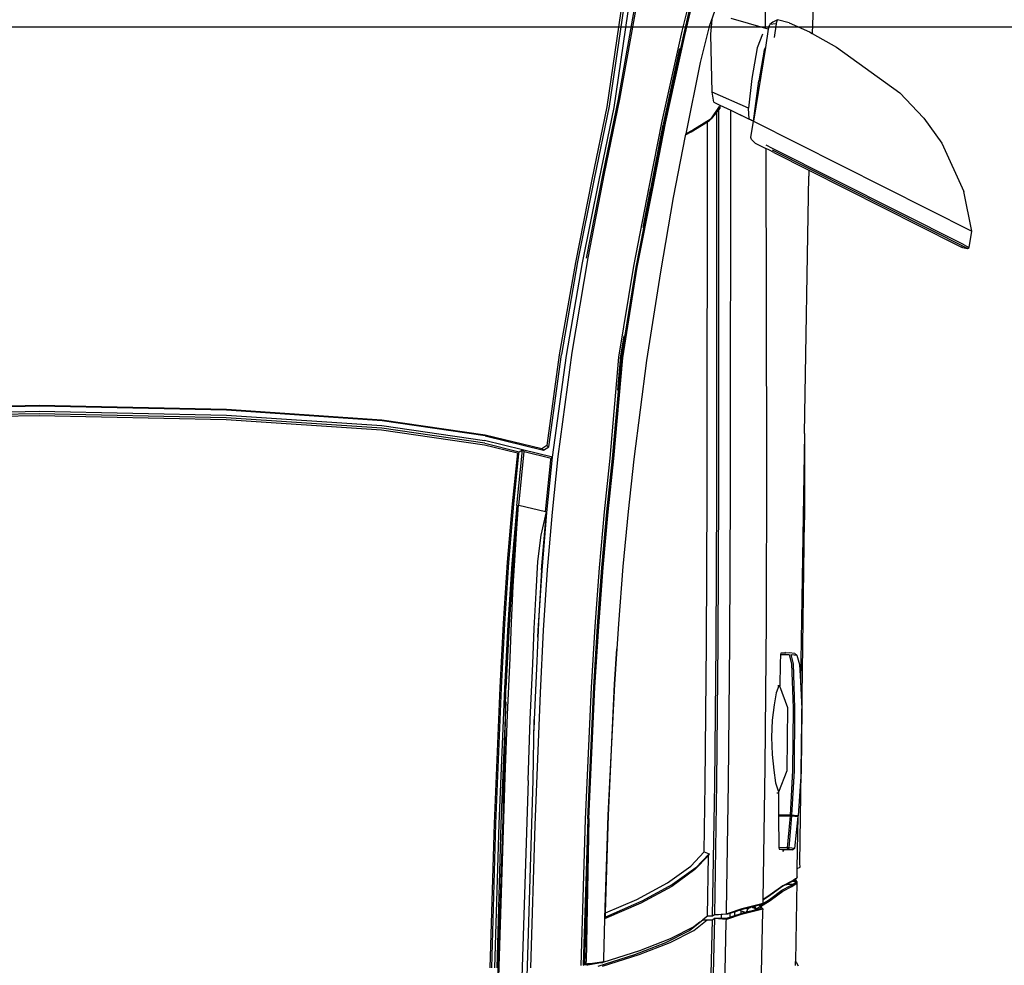
# Model space of a CAD drawing. Units: inches. Extents: x 1319 to 2030, y 219 to 1069.
# Tile 12 of 28: x 1461 to 1506, y 430 to 473. Entities that reach past the tile are written whole.
import ezdxf

# ---------------------------------------------------------------- set-up
doc = ezdxf.new("R2010")
doc.units = ezdxf.units.IN
doc.header["$MEASUREMENT"] = 0
doc.layers.get('0').update_dxf_attribs({"color": 12})
doc.layers.add('A-ANNO-DIMS', color=2, linetype='Continuous', lineweight=18)
doc.layers.add('C-PRKG-VEHC', color=8, linetype='Continuous', lineweight=13)
doc.layers.add('Edges', color=250, linetype='Continuous')
doc.styles.get("Standard").update_dxf_attribs({"font": 'arial.ttf'})
doc.dimstyles.get("Standard").update_dxf_attribs({"dimtxt": 7, "dimasz": 0.18, "dimexe": 0.18, "dimexo": 0.0625, "dimgap": 0.09, "dimtad": 0, "dimtih": 1, "dimtoh": 1, "dimzin": 0, "dimdsep": 46, "dimlunit": 3, "dimtxsty": 'Standard', "dimcen": 0.09, "dimadec": 0, "dimazin": 0, "dimtfac": 1, "dimtofl": 0, "dimtmove": 0, "dimatfit": 3, "dimfxl": 1, "dimtolj": 1, "dimtzin": 0, "dimarcsym": 0})

# ---------------------------------------------------------------- blocks, each defined once
blk = doc.blocks.new('Nissan Qashqai pl')
at = {"layer": 'Edges'}
for p, q in [((8.8918, 12.7444), (9.0186, 12.9956)), ((9.0386, 12.9907), (8.9254, 12.7664)), ((9.0186, 12.9956), (8.9731, 12.9865)), ((9.0374, 12.9925), (9.0186, 12.9956)), ((9.0356, 12.9888), (9.0374, 12.9925)), ((9.0386, 12.9907), (9.0374, 12.9925)), ((9.0376, 12.985), (9.0386, 12.9907)), ((8.9173, 12.961), (8.9731, 12.9865)), ((9.0333, 12.9845), (8.9232, 12.7662)), ((8.9483, 12.8082), (9.0343, 12.9785)), ((9.0356, 12.9888), (9.0333, 12.9845)), ((9.0343, 12.9785), (9.0347, 12.9794)), ((9.0347, 12.9794), (9.0362, 12.9822)), ((9.0362, 12.9822), (9.037, 12.9838)), ((9.0371, 12.9841), (9.037, 12.9838)), ((9.0371, 12.9841), (9.0376, 12.985)), ((9.0376, 12.985), (9.0371, 12.9847)), ((8.8885, 12.9405), (8.9173, 12.961)), ((8.8591, 12.9127), (8.8879, 12.94)), ((8.8885, 12.9405), (8.8879, 12.94)), ((8.8066, 12.84), (8.8591, 12.9127)), ((8.7908, 12.812), (8.8066, 12.84)), ((8.7222, 12.8144), (8.7908, 12.812)), ((8.7785, 12.7855), (8.7891, 12.8089)), ((8.7891, 12.8089), (8.7908, 12.812)), ((8.928, 12.7679), (8.9483, 12.8082)), ((8.9483, 12.8082), (8.9552, 12.8081)), ((9.2517, 12.8031), (8.9552, 12.8081)), ((9.2517, 12.8031), (9.351, 12.803)), ((9.2517, 12.8031), (9.5372, 12.7983)), ((9.641, 12.7991), (9.351, 12.803)), ((9.5069, 12.7941), (9.5176, 12.7972)), ((9.5176, 12.7972), (9.5372, 12.7983)), ((9.5372, 12.7983), (9.5689, 12.7999)), ((9.5689, 12.7999), (9.641, 12.7991)), ((9.641, 12.7991), (9.6921, 12.7956)), ((9.7466, 12.7978), (9.641, 12.7991)), ((9.7511, 12.7979), (9.7466, 12.7978)), ((9.7526, 12.7946), (9.7511, 12.7979)), ((9.5052, 12.7918), (9.5044, 12.7856)), ((9.5052, 12.7918), (9.5069, 12.7941)), ((9.5061, 12.7878), (9.5069, 12.7941)), ((9.5168, 12.7904), (9.5061, 12.7878)), ((9.5061, 12.7856), (9.5167, 12.7883)), ((9.5167, 12.7883), (9.5679, 12.7899)), ((9.5679, 12.792), (9.5168, 12.7904)), ((9.6401, 12.7914), (9.5679, 12.792)), ((9.5679, 12.7899), (9.64, 12.7892)), ((9.64, 12.7892), (9.6912, 12.7865)), ((9.6913, 12.7886), (9.6401, 12.7914)), ((9.6913, 12.7886), (9.6912, 12.7865)), ((9.6912, 12.7865), (9.6912, 12.7811)), ((9.692, 12.7943), (9.6913, 12.7886)), ((9.6921, 12.7956), (9.692, 12.7943)), ((9.6922, 12.7943), (9.692, 12.7943)), ((9.692, 12.7811), (9.6921, 12.7864)), ((9.6922, 12.7943), (9.6921, 12.7956)), ((9.7526, 12.7946), (9.6921, 12.7956)), ((9.6922, 12.7885), (9.6921, 12.7864)), ((9.6921, 12.7864), (9.7288, 12.7832)), ((9.6922, 12.7885), (9.693, 12.7955)), ((9.6922, 12.7885), (9.6922, 12.7943)), ((9.7288, 12.7854), (9.6922, 12.7885)), ((9.693, 12.7955), (9.7296, 12.7914)), ((9.7296, 12.7914), (9.7288, 12.7854)), ((9.7296, 12.7914), (9.7314, 12.7895)), ((9.7306, 12.7834), (9.7314, 12.7895)), ((9.7314, 12.7895), (9.7313, 12.7798)), ((9.7623, 12.7945), (9.7526, 12.7946)), ((9.7623, 12.7945), (9.7643, 12.7937)), ((9.7643, 12.7937), (9.7652, 12.7927)), ((9.7643, 12.7937), (9.7648, 12.7929)), ((9.7648, 12.7929), (9.7648, 12.7929)), ((9.7648, 12.7929), (9.7664, 12.7902)), ((9.7652, 12.7927), (9.7665, 12.7907)), ((9.7665, 12.7904), (9.7664, 12.7902)), ((9.7664, 12.7902), (9.7674, 12.7885)), ((9.7667, 12.7933), (9.7665, 12.7907)), ((9.7665, 12.7907), (9.7676, 12.7889)), ((9.7677, 12.7944), (9.7667, 12.7933)), ((9.7676, 12.7931), (9.7667, 12.7933)), ((9.7673, 12.7899), (9.7676, 12.7931)), ((9.7673, 12.7897), (9.7673, 12.7899)), ((9.7673, 12.7897), (9.7676, 12.7889)), ((9.7674, 12.7885), (9.7728, 12.7781)), ((9.769, 12.7926), (9.7676, 12.7931)), ((9.7676, 12.7889), (9.7684, 12.7875)), ((9.7676, 12.7887), (9.7678, 12.7882)), ((9.7677, 12.7944), (9.7677, 12.7944)), ((9.77, 12.7936), (9.7677, 12.7944)), ((9.7677, 12.7944), (9.8598, 12.7928)), ((9.7684, 12.7875), (9.7717, 12.781)), ((9.7712, 12.7892), (9.769, 12.7926)), ((9.7734, 12.7884), (9.77, 12.7936)), ((9.7707, 12.7848), (9.7709, 12.7893)), ((9.7709, 12.7893), (9.7712, 12.7892)), ((9.7724, 12.7874), (9.7712, 12.7892)), ((9.7778, 12.777), (9.7724, 12.7874)), ((9.7788, 12.778), (9.7734, 12.7884)), ((9.8598, 12.7928), (9.8614, 12.7937)), ((9.8643, 12.7927), (9.8598, 12.7928)), ((9.8614, 12.7937), (9.8647, 12.7956)), ((8.7785, 12.7855), (8.7751, 12.7719)), ((9.5037, 12.7806), (9.5045, 12.7814)), ((9.5044, 12.7856), (9.5045, 12.7814)), ((9.5045, 12.7814), (9.5045, 12.7759)), ((9.5045, 12.7759), (9.5063, 12.7755)), ((9.5063, 12.7755), (9.5061, 12.7856)), ((9.5063, 12.7755), (9.5168, 12.7751)), ((9.5168, 12.7751), (9.5423, 12.7746)), ((9.5423, 12.7746), (9.5422, 12.7736)), ((9.5426, 12.7747), (9.5423, 12.7746)), ((9.5426, 12.7747), (9.5424, 12.7735)), ((9.5678, 12.7837), (9.5426, 12.7747)), ((9.64, 12.7831), (9.5678, 12.7837)), ((9.6645, 12.7737), (9.64, 12.7831)), ((9.6912, 12.7811), (9.6911, 12.7796)), ((9.6911, 12.7796), (9.6911, 12.7732)), ((9.692, 12.7811), (9.6912, 12.7811)), ((9.692, 12.7796), (9.692, 12.7811)), ((9.692, 12.7733), (9.692, 12.7796)), ((9.7288, 12.7832), (9.7287, 12.7734)), ((9.7306, 12.7834), (9.7288, 12.7854)), ((9.7288, 12.7854), (9.7288, 12.7832)), ((9.7288, 12.7832), (9.7306, 12.7834)), ((9.7305, 12.7738), (9.7306, 12.7834)), ((9.7305, 12.7738), (9.7313, 12.7798)), ((9.733, 12.7782), (9.7313, 12.7798)), ((9.7717, 12.781), (9.7707, 12.7848)), ((9.7717, 12.781), (9.7738, 12.7771)), ((9.7728, 12.7781), (9.7832, 12.7637)), ((9.7738, 12.7771), (9.7842, 12.7627)), ((9.7883, 12.7626), (9.7778, 12.777)), ((9.7894, 12.7636), (9.7788, 12.778)), ((8.7751, 12.7719), (8.7779, 12.7668)), ((8.7798, 12.7703), (8.7751, 12.7719)), ((8.7779, 12.7668), (8.7807, 12.763)), ((8.7798, 12.7703), (8.7807, 12.763)), ((8.7798, 12.7703), (8.7954, 12.7683)), ((8.7849, 12.7615), (8.7807, 12.763)), ((8.9232, 12.7662), (8.9194, 12.7588)), ((8.928, 12.7679), (8.925, 12.762)), ((9.5422, 12.7736), (9.5422, 12.7725)), ((9.5422, 12.7736), (9.5424, 12.7735)), ((9.5424, 12.7735), (9.5503, 12.7706)), ((9.5503, 12.7706), (9.5641, 12.7681)), ((9.5641, 12.7681), (9.5818, 12.766)), ((9.5818, 12.766), (9.6016, 12.7651)), ((9.6016, 12.7651), (9.6215, 12.766)), ((9.6215, 12.766), (9.6395, 12.7676)), ((9.6395, 12.7676), (9.654, 12.7697)), ((9.654, 12.7697), (9.6633, 12.7726)), ((9.6633, 12.7726), (9.6645, 12.7737)), ((9.6655, 12.7733), (9.6645, 12.7737)), ((9.6655, 12.7733), (9.6911, 12.7732)), ((9.6655, 12.7713), (9.6655, 12.7733)), ((9.6911, 12.7732), (9.692, 12.7733)), ((9.692, 12.7733), (9.7287, 12.7734)), ((9.7287, 12.7734), (9.7305, 12.7738)), ((9.7832, 12.7637), (9.7887, 12.7552)), ((9.7965, 12.7526), (9.7894, 12.7636)), ((8.7849, 12.7582), (8.7205, 12.7579)), ((8.7734, 12.7181), (8.7849, 12.7582)), ((8.7849, 12.7615), (8.7858, 12.7613)), ((8.7849, 12.7582), (8.7856, 12.7608)), ((8.7858, 12.7613), (8.7856, 12.7608)), ((8.7858, 12.7613), (8.807, 12.758)), ((8.7917, 12.7547), (8.8075, 12.7486)), ((8.8102, 12.7568), (8.807, 12.758)), ((8.807, 12.758), (8.8918, 12.7444)), ((8.8102, 12.7568), (8.8455, 12.7506)), ((8.9171, 12.7464), (8.9233, 12.7586)), ((8.925, 12.762), (8.9233, 12.7586)), ((8.9233, 12.7586), (9.2886, 12.7594)), ((9.2886, 12.7594), (9.4673, 12.7589)), ((9.4673, 12.7589), (9.6358, 12.7575)), ((9.6358, 12.7575), (9.7887, 12.7552)), ((9.7842, 12.7627), (9.7891, 12.7552)), ((9.7933, 12.7549), (9.7883, 12.7626)), ((9.7887, 12.7552), (9.7891, 12.7552)), ((9.7891, 12.7552), (9.79, 12.7552)), ((9.79, 12.7552), (9.7931, 12.7552)), ((9.7931, 12.7552), (9.7934, 12.7535)), ((9.7931, 12.7552), (9.7933, 12.7549)), ((9.7933, 12.7549), (9.7941, 12.7541)), ((9.7934, 12.7535), (9.7938, 12.7538)), ((9.7934, 12.7535), (9.7937, 12.7524)), ((9.7937, 12.7524), (9.7992, 12.7308)), ((9.7941, 12.7541), (9.7943, 12.7535)), ((9.7955, 12.7516), (9.7943, 12.7535)), ((9.7943, 12.7535), (9.7964, 12.7453)), ((9.7963, 12.7523), (9.7955, 12.7516)), ((9.7963, 12.7523), (9.7963, 12.7524)), ((9.7964, 12.7524), (9.7963, 12.7523)), ((9.7992, 12.7476), (9.7963, 12.7523)), ((9.7967, 12.7526), (9.7964, 12.7524)), ((9.7964, 12.7525), (9.7964, 12.7524)), ((9.7964, 12.7524), (9.7996, 12.7475)), ((9.7983, 12.7541), (9.7965, 12.7526)), ((9.7965, 12.7526), (9.7967, 12.7526)), ((9.7977, 12.7535), (9.7967, 12.7526)), ((9.7967, 12.7526), (9.7986, 12.7526)), ((9.7982, 12.754), (9.7977, 12.7535)), ((9.7983, 12.7541), (9.7982, 12.754)), ((9.7986, 12.7526), (9.7982, 12.754)), ((9.7986, 12.7544), (9.7983, 12.7541)), ((9.7993, 12.755), (9.7986, 12.7544)), ((9.7988, 12.7516), (9.7986, 12.7526)), ((9.7998, 12.7477), (9.7988, 12.7516)), ((9.7999, 12.7522), (9.7993, 12.755)), ((9.7993, 12.755), (9.8024, 12.7549)), ((9.8054, 12.7307), (9.7999, 12.7522)), ((9.8024, 12.7549), (9.9426, 12.7518)), ((8.8075, 12.7486), (8.8429, 12.7426)), ((8.8429, 12.7426), (8.8771, 12.7388)), ((8.8918, 12.7444), (8.8455, 12.7506)), ((8.8815, 12.7228), (8.892, 12.7444)), ((8.8908, 12.7421), (8.8895, 12.7393)), ((8.8906, 12.7418), (8.8895, 12.7393)), ((8.8906, 12.7418), (8.8911, 12.7428)), ((8.892, 12.7444), (8.8908, 12.7421)), ((8.8911, 12.7428), (8.8919, 12.7444)), ((8.8911, 12.7428), (8.8919, 12.7444)), ((8.8919, 12.7444), (8.8911, 12.7428)), ((8.8919, 12.7444), (8.8918, 12.7444)), ((8.892, 12.7444), (8.8919, 12.7444)), ((8.8919, 12.7444), (8.8919, 12.7444)), ((8.8919, 12.7444), (8.8919, 12.7444)), ((8.9106, 12.7413), (8.892, 12.7444)), ((8.892, 12.7444), (8.892, 12.7444)), ((8.9131, 12.7421), (8.9106, 12.7413)), ((8.9171, 12.7464), (8.9131, 12.7421)), ((8.9171, 12.7464), (8.917, 12.7468)), ((9.7964, 12.7453), (9.7992, 12.7476)), ((9.7964, 12.7453), (9.7973, 12.7418)), ((9.7977, 12.7431), (9.7973, 12.7418)), ((9.7973, 12.7418), (9.7977, 12.7409)), ((9.7973, 12.7418), (9.7977, 12.7399)), ((9.7977, 12.7444), (9.7985, 12.7451)), ((9.7985, 12.7451), (9.7977, 12.7431)), ((9.7977, 12.7431), (9.7977, 12.7444)), ((9.7977, 12.7399), (9.7977, 12.7409)), ((9.7977, 12.7409), (9.7987, 12.7388)), ((9.7989, 12.7461), (9.7985, 12.7451)), ((9.7998, 12.7466), (9.7989, 12.7461)), ((9.7998, 12.7466), (9.7992, 12.7476)), ((9.7996, 12.7475), (9.7998, 12.7477)), ((9.8002, 12.7461), (9.7996, 12.7475)), ((9.8001, 12.7468), (9.7996, 12.7475)), ((9.8001, 12.7468), (9.7998, 12.7477)), ((9.8003, 12.7458), (9.7998, 12.7466)), ((9.8002, 12.7461), (9.8001, 12.7468)), ((9.8003, 12.7458), (9.8002, 12.7461)), ((9.8027, 12.7364), (9.8003, 12.7458)), ((8.8771, 12.7388), (8.8585, 12.6969)), ((8.8895, 12.7393), (8.8771, 12.7388)), ((8.8815, 12.7228), (8.8895, 12.7393)), ((9.7977, 12.7399), (9.7978, 12.7397)), ((9.7987, 12.7388), (9.7978, 12.7397)), ((9.7978, 12.7397), (9.7987, 12.7362)), ((9.7987, 12.7388), (9.7992, 12.7377)), ((9.7987, 12.7362), (9.7992, 12.7377)), ((9.7987, 12.7362), (9.8002, 12.7301)), ((9.7992, 12.7377), (9.8027, 12.7364)), ((9.7992, 12.7308), (9.8044, 12.7151)), ((9.8002, 12.7301), (9.8008, 12.7285)), ((9.8008, 12.7285), (9.8014, 12.7303)), ((9.8014, 12.7303), (9.8031, 12.7349)), ((9.8043, 12.7303), (9.8014, 12.7303)), ((9.8031, 12.7349), (9.8027, 12.7364)), ((9.8043, 12.7303), (9.8031, 12.7349)), ((9.8044, 12.73), (9.8043, 12.7303)), ((9.8067, 12.7229), (9.8044, 12.73)), ((9.8106, 12.715), (9.8054, 12.7307)), ((8.8734, 12.7057), (8.8793, 12.7181)), ((8.8793, 12.7181), (8.8815, 12.7228)), ((9.3194, 12.7179), (8.8793, 12.7181)), ((9.4919, 12.7173), (9.3194, 12.7179)), ((9.8008, 12.7285), (9.8014, 12.7265)), ((9.8014, 12.7265), (9.803, 12.723)), ((9.8014, 12.7265), (9.8026, 12.723)), ((9.803, 12.723), (9.8026, 12.723)), ((9.8026, 12.723), (9.8046, 12.7171)), ((9.8067, 12.7229), (9.803, 12.723)), ((9.8086, 12.7171), (9.8067, 12.7229)), ((9.6538, 12.7157), (9.4919, 12.7173)), ((9.802, 12.7133), (9.6538, 12.7157)), ((9.8051, 12.7132), (9.802, 12.7133)), ((9.8044, 12.7151), (9.8051, 12.7132)), ((9.8046, 12.7171), (9.8086, 12.7171)), ((9.8046, 12.7171), (9.8055, 12.7143)), ((9.8061, 12.6994), (9.8051, 12.7132)), ((9.8055, 12.7143), (9.8058, 12.7073)), ((9.8058, 12.7073), (9.8098, 12.7073)), ((9.8058, 12.7073), (9.8061, 12.6994)), ((9.8096, 12.7142), (9.8086, 12.7171)), ((9.8098, 12.7073), (9.8096, 12.7142)), ((9.8101, 12.6993), (9.8098, 12.7073)), ((9.8101, 12.6993), (9.8112, 12.7131)), ((9.8112, 12.7131), (9.8106, 12.715)), ((9.8143, 12.713), (9.8112, 12.7131)), ((9.9414, 12.71), (9.8143, 12.713)), ((8.7524, 12.704), (8.7828, 12.6934)), ((8.7916, 12.6954), (8.7748, 12.6967)), ((8.8259, 12.6959), (8.7916, 12.6954)), ((8.8585, 12.6969), (8.8259, 12.6959)), ((8.87, 12.6987), (8.8585, 12.6969)), ((8.87, 12.6987), (8.8734, 12.7057)), ((8.8734, 12.7057), (8.8768, 12.7057)), ((8.8751, 12.7054), (8.8768, 12.7057)), ((8.8893, 12.6956), (8.8751, 12.7054)), ((8.8768, 12.7057), (8.879, 12.704)), ((8.879, 12.704), (9.3198, 12.7039)), ((8.879, 12.704), (8.881, 12.7023)), ((9.3225, 12.7021), (8.881, 12.7023)), ((8.881, 12.7023), (8.8893, 12.6956)), ((8.8893, 12.6956), (8.9021, 12.6745)), ((8.8913, 12.6936), (8.8893, 12.6956)), ((9.3198, 12.7039), (9.4922, 12.7033)), ((9.4936, 12.7013), (9.3225, 12.7021)), ((9.4922, 12.7033), (9.654, 12.7018)), ((9.6552, 12.6997), (9.4936, 12.7013)), ((9.654, 12.7018), (9.8061, 12.6994)), ((9.8078, 12.6971), (9.6552, 12.6997)), ((9.8061, 12.6994), (9.8078, 12.6971)), ((9.8078, 12.6971), (9.8078, 12.6913)), ((9.8119, 12.697), (9.8101, 12.6993)), ((9.8101, 12.6993), (9.9411, 12.6966)), ((9.9393, 12.6944), (9.8119, 12.697)), ((9.8119, 12.6912), (9.8119, 12.697)), ((8.7828, 12.6934), (8.8245, 12.6828)), ((8.8927, 12.6913), (8.8913, 12.6936)), ((9.3224, 12.6911), (8.8927, 12.6913)), ((8.9041, 12.6725), (8.8927, 12.6913)), ((9.3225, 12.6911), (9.3224, 12.6911)), ((9.4936, 12.6904), (9.3225, 12.6911)), ((9.6552, 12.6888), (9.4936, 12.6904)), ((9.7337, 12.6875), (9.6552, 12.6888)), ((9.7337, 12.6875), (9.7357, 12.6935)), ((9.7499, 12.6721), (9.7337, 12.6875)), ((9.7357, 12.6935), (9.7378, 12.6924)), ((9.7357, 12.6935), (9.7519, 12.678)), ((9.7378, 12.6924), (9.754, 12.677)), ((9.8078, 12.6913), (9.7378, 12.6924)), ((9.8078, 12.6913), (9.8119, 12.6862)), ((9.8241, 12.6756), (9.8119, 12.6912)), ((9.8119, 12.6862), (9.8119, 12.6912)), ((9.8147, 12.6826), (9.8119, 12.6862)), ((8.7931, 12.6653), (8.7574, 12.6737)), ((8.8245, 12.6828), (8.9063, 12.6663)), ((8.9021, 12.6745), (8.9063, 12.6663)), ((8.9075, 12.6661), (8.9041, 12.6725)), ((9.7519, 12.678), (9.7713, 12.6512)), ((9.754, 12.677), (9.7733, 12.6502)), ((9.8147, 12.6826), (9.8147, 12.6826)), ((9.8147, 12.6826), (9.8201, 12.6756)), ((9.8241, 12.6706), (9.8147, 12.6826)), ((9.8201, 12.6756), (9.8338, 12.6486)), ((9.8378, 12.6485), (9.8241, 12.6756)), ((8.7881, 12.6621), (8.7575, 12.6698)), ((8.7925, 12.664), (8.7591, 12.6719)), ((8.8918, 12.6392), (8.7881, 12.6621)), ((8.8941, 12.6418), (8.7925, 12.664)), ((8.8942, 12.6432), (8.7931, 12.6653)), ((8.9063, 12.6663), (8.9075, 12.6661)), ((8.9075, 12.6661), (8.9087, 12.6658)), ((8.9087, 12.6658), (8.9797, 12.6518)), ((9.7692, 12.6453), (9.7499, 12.6721)), ((9.8378, 12.6435), (9.8241, 12.6706)), ((8.8083, 12.6591), (8.8954, 12.6403)), ((8.9797, 12.6518), (9.0656, 12.6372)), ((9.7713, 12.6512), (9.7905, 12.6158)), ((9.7733, 12.6502), (9.7925, 12.6148)), ((8.9679, 12.6241), (8.8918, 12.6392)), ((9.0601, 12.6092), (8.8941, 12.6418)), ((8.9696, 12.6285), (8.8942, 12.6432)), ((8.8961, 12.6401), (8.9704, 12.6257)), ((9.7885, 12.6099), (9.7692, 12.6453)), ((9.8338, 12.6486), (9.8475, 12.613)), ((9.8516, 12.6129), (9.8378, 12.6485)), ((9.8516, 12.6079), (9.8378, 12.6435)), ((9.06, 12.6106), (8.9696, 12.6285)), ((9.0656, 12.6372), (9.1676, 12.6212)), ((9.0591, 12.6065), (8.9679, 12.6241)), ((8.9704, 12.6257), (8.9708, 12.6256)), ((8.9708, 12.6256), (9.0143, 12.6169)), ((9.1676, 12.6212), (9.2814, 12.6065)), ((9.7905, 12.6158), (9.8087, 12.574)), ((8.8666, 12.5888), (8.7287, 12.6134)), ((8.7292, 12.6146), (8.8666, 12.5901)), ((9.1639, 12.5895), (9.0591, 12.6065)), ((9.1644, 12.5938), (9.06, 12.6106)), ((9.1645, 12.5924), (9.0601, 12.6092)), ((9.2814, 12.6065), (9.3416, 12.5999)), ((9.8039, 12.5741), (9.7885, 12.6099)), ((9.7925, 12.6148), (9.8107, 12.573)), ((9.8475, 12.613), (9.8611, 12.5708)), ((9.8652, 12.5704), (9.8516, 12.6129)), ((9.8652, 12.5654), (9.8516, 12.6079)), ((8.7481, 12.5968), (8.8745, 12.5782)), ((8.7491, 12.594), (8.8754, 12.5755)), ((8.8761, 12.5839), (8.7496, 12.6025)), ((9.1393, 12.5951), (9.1647, 12.591)), ((9.2803, 12.5836), (9.1644, 12.5938)), ((9.3416, 12.5999), (9.4048, 12.5941)), ((9.4048, 12.5941), (9.471, 12.5888)), ((8.8666, 12.5901), (8.9521, 12.5726)), ((8.9522, 12.5713), (8.8666, 12.5888)), ((8.9598, 12.5666), (8.8761, 12.5839)), ((9.2801, 12.5794), (9.1639, 12.5895)), ((9.2804, 12.5821), (9.1645, 12.5924)), ((9.1647, 12.591), (9.1668, 12.5908)), ((9.1668, 12.5908), (9.2019, 12.5877)), ((9.3418, 12.5771), (9.2803, 12.5836)), ((9.3419, 12.5756), (9.2804, 12.5821)), ((9.471, 12.5888), (9.4997, 12.5869)), ((9.5404, 12.5844), (9.4997, 12.5869)), ((9.4997, 12.5869), (9.5403, 12.5842)), ((9.5403, 12.5842), (9.6913, 12.5767)), ((9.6912, 12.5774), (9.5404, 12.5844)), ((8.8745, 12.5782), (8.9583, 12.5609)), ((8.8754, 12.5755), (8.9591, 12.5583)), ((8.9521, 12.5726), (9.0495, 12.5536)), ((9.0497, 12.5523), (8.9522, 12.5713)), ((9.3418, 12.5729), (9.2801, 12.5794)), ((9.4062, 12.5713), (9.3418, 12.5771)), ((9.4064, 12.5671), (9.3418, 12.5729)), ((9.4063, 12.5699), (9.3419, 12.5756)), ((9.4735, 12.5663), (9.4062, 12.5713)), ((9.8039, 12.5741), (9.6912, 12.5774)), ((9.6913, 12.5767), (9.8099, 12.573)), ((9.8087, 12.574), (9.8039, 12.5741)), ((9.8099, 12.573), (9.8087, 12.574)), ((9.8099, 12.573), (9.8107, 12.573)), ((9.8107, 12.573), (9.8573, 12.5716)), ((9.8573, 12.5716), (9.8603, 12.5715)), ((9.8603, 12.5715), (9.8605, 12.5696)), ((9.8611, 12.5708), (9.8603, 12.5715)), ((9.8612, 12.5707), (9.8611, 12.5708)), ((9.8612, 12.5707), (9.8615, 12.5688)), ((8.9583, 12.5609), (9.0538, 12.5419)), ((9.0552, 12.5477), (8.9598, 12.5666)), ((9.4736, 12.5648), (9.4063, 12.5699)), ((9.4739, 12.5621), (9.4064, 12.5671)), ((9.5437, 12.5619), (9.4735, 12.5663)), ((9.5438, 12.5605), (9.4736, 12.5648)), ((9.5443, 12.5579), (9.4739, 12.5621)), ((9.6953, 12.5549), (9.5437, 12.5619)), ((9.6954, 12.5535), (9.5438, 12.5605)), ((9.8605, 12.5696), (9.8626, 12.5564)), ((9.8615, 12.5688), (9.8635, 12.5556)), ((8.9591, 12.5583), (9.0546, 12.5394)), ((9.0495, 12.5536), (9.1584, 12.5351)), ((9.1617, 12.5292), (9.0552, 12.5477)), ((9.696, 12.551), (9.5443, 12.5579)), ((9.6953, 12.5549), (9.8598, 12.5517)), ((9.6953, 12.5549), (9.863, 12.5497)), ((9.6954, 12.5535), (9.8641, 12.5483)), ((9.8644, 12.5459), (9.696, 12.551)), ((9.8629, 12.5516), (9.8598, 12.5517)), ((9.8626, 12.5564), (9.8627, 12.5532)), ((9.8637, 12.5532), (9.8627, 12.5532)), ((9.8627, 12.5532), (9.8629, 12.5516)), ((9.8629, 12.5516), (9.863, 12.5497)), ((9.8641, 12.5483), (9.863, 12.5497)), ((9.8635, 12.5556), (9.8637, 12.5532)), ((9.8643, 12.5532), (9.8637, 12.5532)), ((9.8637, 12.5532), (9.8638, 12.5508)), ((9.8638, 12.5508), (9.8641, 12.5483)), ((9.0538, 12.5419), (9.1605, 12.5233)), ((9.0546, 12.5394), (9.1612, 12.5208)), ((9.1584, 12.5351), (9.2783, 12.5191)), ((9.2789, 12.5131), (9.1617, 12.5292)), ((9.2669, 12.5088), (9.1605, 12.5233)), ((9.1612, 12.5208), (9.2656, 12.5065)), ((9.2783, 12.5191), (9.3422, 12.5126)), ((9.2543, 12.4356), (9.2707, 12.5028)), ((9.2656, 12.5065), (9.2669, 12.5088)), ((9.2656, 12.5065), (9.2694, 12.5006)), ((9.2707, 12.5028), (9.2669, 12.5088)), ((9.2707, 12.5028), (9.2694, 12.5006)), ((9.2789, 12.5131), (9.2704, 12.4783)), ((9.2724, 12.4804), (9.2799, 12.5114)), ((9.2799, 12.5114), (9.2789, 12.5131)), ((9.3427, 12.5066), (9.2789, 12.5131)), ((9.2819, 12.5112), (9.2799, 12.5114)), ((9.2803, 12.5116), (9.2822, 12.5118)), ((9.3418, 12.5051), (9.2819, 12.5112)), ((9.3418, 12.5051), (9.3346, 12.4741)), ((9.342, 12.5059), (9.3418, 12.5051)), ((9.3687, 12.5), (9.342, 12.5059)), ((9.4087, 12.5003), (9.342, 12.5059)), ((9.3422, 12.5126), (9.4088, 12.507)), ((9.4093, 12.5011), (9.3427, 12.5066)), ((9.4088, 12.507), (9.4782, 12.5024)), ((9.4782, 12.5024), (9.5503, 12.4987)), ((9.2694, 12.5006), (9.2535, 12.4354)), ((9.3992, 12.496), (9.3687, 12.5)), ((9.4347, 12.494), (9.3992, 12.496)), ((9.4087, 12.5003), (9.4688, 12.4968)), ((9.4785, 12.4965), (9.4093, 12.5011)), ((9.4761, 12.4919), (9.4347, 12.494)), ((9.4688, 12.4968), (9.4789, 12.4964)), ((9.5168, 12.4903), (9.4761, 12.4919)), ((9.4789, 12.4964), (9.4785, 12.4965)), ((9.4862, 12.4961), (9.4785, 12.4965)), ((9.4789, 12.4964), (9.4862, 12.4961)), ((9.4862, 12.4961), (9.514, 12.4949)), ((9.514, 12.4949), (9.5811, 12.492)), ((9.5503, 12.4987), (9.7029, 12.4926)), ((9.651, 12.4906), (9.5811, 12.492)), ((9.5811, 12.492), (9.594, 12.4914)), ((9.7029, 12.4926), (9.8673, 12.4878)), ((9.2724, 12.4804), (9.2704, 12.4783)), ((9.3346, 12.4741), (9.2724, 12.4804)), ((9.5812, 12.4874), (9.5168, 12.4903)), ((9.6514, 12.4849), (9.5812, 12.4874)), ((9.9583, 12.4812), (9.651, 12.4906)), ((9.6514, 12.4849), (9.9312, 12.4761)), ((9.2704, 12.4783), (9.2598, 12.4348)), ((9.2629, 12.435), (9.2726, 12.4746)), ((9.2649, 12.4348), (9.2741, 12.4725)), ((9.2726, 12.4746), (9.2704, 12.4783)), ((9.3346, 12.4718), (9.2704, 12.4783)), ((9.2746, 12.4744), (9.2726, 12.4746)), ((9.2741, 12.4725), (9.3326, 12.4666)), ((9.333, 12.4685), (9.2746, 12.4744)), ((9.4004, 12.4629), (9.333, 12.4685)), ((9.3346, 12.4741), (9.3344, 12.4733)), ((9.3344, 12.4733), (9.4017, 12.4677)), ((9.3344, 12.4733), (9.3611, 12.4715)), ((9.3346, 12.4718), (9.4018, 12.4661)), ((9.3611, 12.4715), (9.3918, 12.4695)), ((9.3918, 12.4695), (9.4276, 12.4674)), ((9.3326, 12.4666), (9.4, 12.4609)), ((9.4, 12.4609), (9.4706, 12.4561)), ((9.4709, 12.4581), (9.4004, 12.4629)), ((9.4017, 12.4677), (9.472, 12.463)), ((9.4018, 12.4661), (9.472, 12.4614)), ((9.4276, 12.4674), (9.4694, 12.4654)), ((9.4694, 12.4654), (9.5105, 12.4637)), ((9.5446, 12.4542), (9.4709, 12.4581)), ((9.472, 12.463), (9.5454, 12.4591)), ((9.472, 12.4614), (9.5454, 12.4576)), ((9.5105, 12.4637), (9.5755, 12.4608)), ((9.5454, 12.4591), (9.5454, 12.4593)), ((9.5695, 12.4589), (9.5454, 12.4591)), ((9.5454, 12.4576), (9.7014, 12.4513)), ((9.5609, 12.4593), (9.5695, 12.4589)), ((9.5786, 12.4588), (9.5695, 12.4589)), ((9.5695, 12.4589), (9.7014, 12.4536)), ((9.5755, 12.4608), (9.6472, 12.4581)), ((9.6206, 12.4581), (9.5786, 12.4588)), ((9.6714, 12.4567), (9.6206, 12.4581)), ((9.6414, 12.458), (9.6407, 12.458)), ((9.6472, 12.4581), (9.9278, 12.4492)), ((9.6549, 12.4576), (9.6558, 12.4574)), ((9.4706, 12.4561), (9.5443, 12.4522)), ((9.5443, 12.4522), (9.701, 12.4459)), ((9.7011, 12.4478), (9.5446, 12.4542)), ((9.6825, 12.4564), (9.6714, 12.4567)), ((9.6825, 12.4564), (9.6829, 12.4563)), ((9.6943, 12.456), (9.6825, 12.4564)), ((9.6943, 12.4558), (9.6943, 12.456)), ((9.6951, 12.456), (9.6943, 12.456)), ((9.6951, 12.4558), (9.6951, 12.456)), ((9.8565, 12.451), (9.6951, 12.456)), ((9.701, 12.4459), (9.8673, 12.441)), ((9.8673, 12.443), (9.7011, 12.4478)), ((9.7014, 12.4536), (9.8673, 12.4488)), ((9.7014, 12.4513), (9.8673, 12.4464)), ((9.9794, 12.4475), (9.8565, 12.451)), ((9.2535, 12.4354), (9.2362, 12.3167)), ((9.2543, 12.4356), (9.2371, 12.3169)), ((9.2426, 12.3164), (9.2598, 12.4348)), ((9.2629, 12.435), (9.2457, 12.3164)), ((9.2476, 12.3163), (9.2649, 12.4348)), ((9.2362, 12.3167), (9.2241, 12.1376)), ((9.2371, 12.3169), (9.2249, 12.1376)), ((9.2305, 12.1375), (9.2426, 12.3164)), ((9.2457, 12.3164), (9.2335, 12.1374)), ((9.2355, 12.1374), (9.2476, 12.3163)), ((9.2241, 12.1376), (9.2195, 11.9221)), ((9.2249, 12.1376), (9.2203, 11.9221)), ((9.2259, 11.9221), (9.2305, 12.1375)), ((9.2335, 12.1374), (9.2289, 11.9221)), ((9.2308, 11.9221), (9.2355, 12.1374)), ((9.2195, 11.9221), (9.2241, 11.7066)), ((9.2203, 11.9221), (9.2249, 11.7065)), ((9.2305, 11.7067), (9.2259, 11.9221)), ((9.2289, 11.9221), (9.2335, 11.7067)), ((9.2355, 11.7068), (9.2308, 11.9221))]:
    blk.add_line(p, q, dxfattribs=at)
blk = doc.blocks.new('car')
blk.add_blockref('Nissan Qashqai pl', (-9.7433, -11.9151))
blk = doc.blocks.new('carr')
blk.add_blockref('car', (0.5124, -0.007))
blk = doc.blocks.new('*D65')
at = {"layer": 'A-ANNO-DIMS', "color": 0, "lineweight": -2, "transparency": 16777216}
for p, q in [((1648.280254, 472.227245), (1329.112754, 472.227245)), ((1329.292754, 472.047245), (1329.292754, 431.817245)), ((1329.292754, 384.407245), (1329.292754, 424.637245)), ((1648.280254, 384.227245), (1329.112754, 384.227245))]:
    blk.add_line(p, q, dxfattribs=at)
at = {"layer": 'A-ANNO-DIMS', "color": 0, "transparency": 16777216}
for points in [[(1329.262754, 472.047245), (1329.322754, 472.047245), (1329.292754, 472.227245)], [(1329.262754, 384.407245), (1329.322754, 384.407245), (1329.292754, 384.227245)]]:
    blk.add_solid(points, dxfattribs=at)
at = {"layer": 'Defpoints', "color": 0, "transparency": 16777216}
for p in [(1329.292754, 472.227245), (1648.342754, 472.227245), (1648.342754, 384.227245)]:
    blk.add_point(p, dxfattribs=at)
at = {"layer": 'A-ANNO-DIMS', "color": 0, "transparency": 16777216, "insert": (1329.292754, 428.227245), "char_height": 7, "attachment_point": 5}
blk.add_mtext('\\A1;7\'-4"', dxfattribs=at)

msp = doc.modelspace()

# ---------------------------------------------------------------- block references
at = {"layer": 'C-PRKG-VEHC', "xscale": 39.37007874015748, "yscale": 39.37007874015748, "zscale": 39.37007874015748, "rotation": 270}
msp.add_blockref('carr', (1462.179, 454.621), dxfattribs=at)

# ---------------------------------------------------------------- dimensions: what is measured, and where the dimension line sits
at = {"layer": 'A-ANNO-DIMS'}
dim = msp.add_linear_dim(base=(1329.293, 472.227), p1=(1648.343, 384.227), p2=(1648.343, 472.227), angle=90, dimstyle='Standard', override={"dimdec": 1, "dimlfac": 1, "dimrnd": 0, "dimzin": 1, "dimdsep": 46, "dimlunit": 4, "dimfrac": 2}, dxfattribs=at)
dim.commit()
dim.dimension.update_dxf_attribs({"geometry": '*D65', "text_midpoint": (1329.293, 428.227)})

doc.saveas('drawing.dxf')
